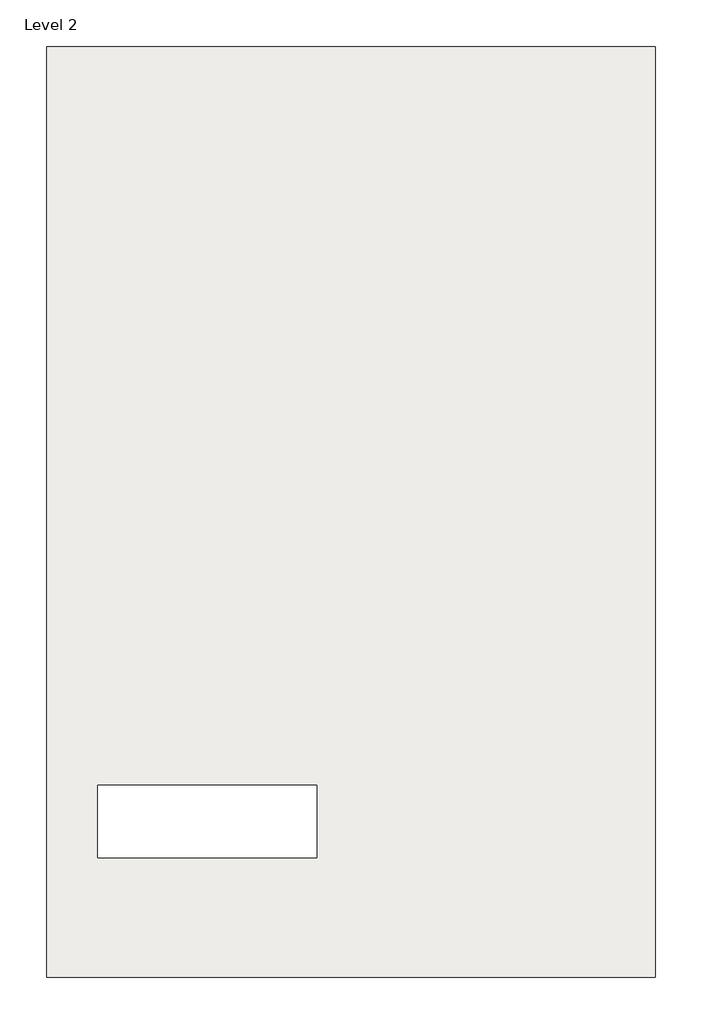
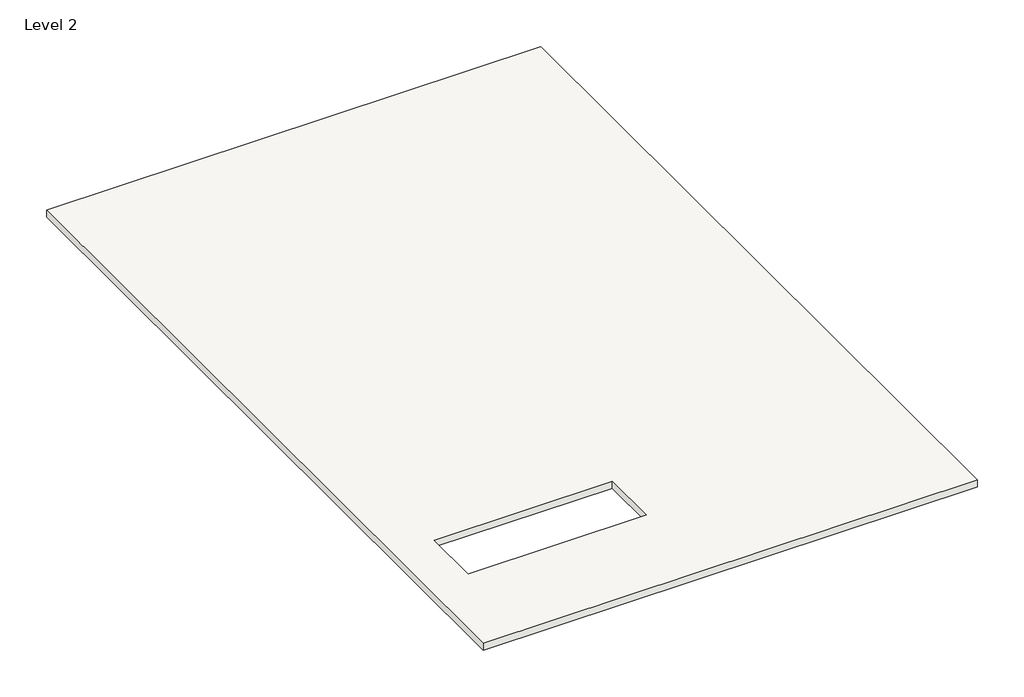
# One storey, incomplete: 1 roof.
"""IFC4 building model written with IfcOpenShell, lengths in millimetres."""

from ifc_helpers import new_model, si_unit, frame, origin, place, context, project, spatial, polyline, outline, extrude, element, save

model = new_model("IFC4")

# Units and contexts
model_context = context("Model", 3, world=origin())
ifc_project = project(units=[si_unit("LENGTHUNIT", "METRE", prefix="MILLI")], contexts=[model_context])

# Site, building, storey
site = spatial("IfcSite", under=ifc_project)
building = spatial("IfcBuilding", under=site)
storey = spatial("IfcBuildingStorey", under=building, Name="Level 2", Elevation=3048.0)

# Roof
placement = place(None, origin())
element("IfcRoof", 1, ObjectType="ROOF 6\"", at=placement, inside=storey, context=model_context, shape_type="SweptSolid", body=[
    extrude(outline(polyline([(-6377.9198569, -8544.8933037), (-6377.9198569, 7126.9066963), (3870.9801431, 7126.9066963), (3870.9801431, -8544.8933037), (-6377.9198569, -8544.8933037)]), holes=[polyline([(-5514.3198569, -5306.3933037), (-5514.3198569, -6525.5933037), (-1831.3198569, -6525.5933037), (-1831.3198569, -5306.3933037), (-5514.3198569, -5306.3933037)])]), frame((0.0, 0.0, 3048.0), z_axis=(0.0, 0.0, 1.0), x_axis=(1.0, 0.0, 0.0)), (0.0, 0.0, 1.0), 152.4),
])

save(model, "model.ifc")

# Revit data of these elements
# Type "ROOF 6\""
#   Assembly Code = "B1020"
#   Layers, outside or top first: 0' - 6" no material (function 1)
# Element 1 (IfcRoof, "ROOF 6\"")
#   built-in parameter 1001705 = 10.5 (stored number, unit not read)
#   built-in parameter 1001710 = 33615
#   Phase Created = New Construction
#   Materials on its faces: "Default Roof", "Parking Stripe", "Wood - Stained"
# Materials
#   "Default Roof": colour RGB 88 101 114, transparency 0, Cost = 0
#   "Parking Stripe": class "Paint", colour RGB 250 250 91, transparency 0, Cost = 0
#   "Wood - Stained": class "Wood", colour RGB 224 178 126, transparency 0, Cost = 0
